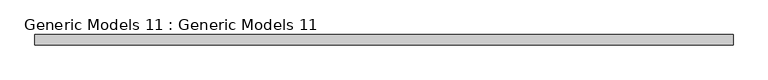
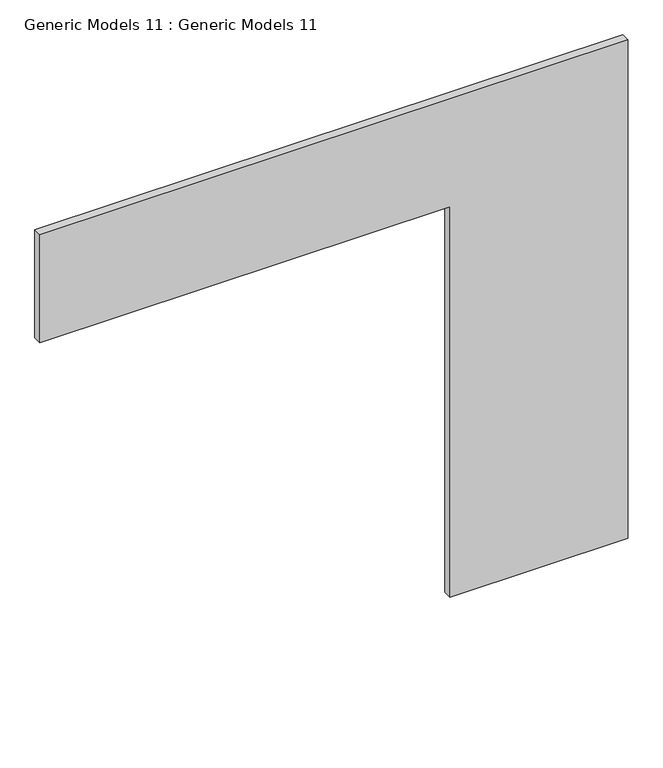
"""IFC4 building model written with IfcOpenShell, lengths in millimetres: proxy geometry, Generic Models 11 : Generic Models 11."""

from ifc_helpers import new_model, si_unit, frame, origin, place, context, project, spatial, polyline, outline, extrude, source, transform, mapped, element, save


def generic_models_11_generic_models_11_47c1f207(model_context):
    return source(origin(), model_context, "Body", "SweptSolid", [
        extrude(outline(polyline([(3352.8, -2406.7607439), (3352.8, -5810.3607439), (2692.4, -5810.3607439), (2692.4, -3435.4607439), (304.8, -3435.4607439), (304.8, -2406.7607439), (2673.920695, -2406.7607439), (3352.8, -2406.7607439)])), frame((0.0, -6621.2842658, 0.0), z_axis=(0.0, 1.0, 0.0), x_axis=(0.0, 0.0, 1.0)), (0.0, 0.0, 1.0), 50.8),
    ])


if __name__ == "__main__":
    model = new_model("IFC4")
    model_context = context("Model", 3, world=origin())
    ifc_project = project(units=[si_unit("LENGTHUNIT", "METRE", prefix="MILLI")], contexts=[model_context])
    site = spatial("IfcSite", under=ifc_project)
    building = spatial("IfcBuilding", under=site)
    placement = place(None, origin())
    generic_models_11_generic_models_11_shape = generic_models_11_generic_models_11_47c1f207(model_context)
    element("IfcBuildingElementProxy", 1, Name="Generic Models 11 : Generic Models 11", ObjectType="Generic Models 11 : Generic Models 11", at=placement, inside=building, context=model_context, shape_type="MappedRepresentation", body=[
        mapped(generic_models_11_generic_models_11_shape, transform((0.0, 0.0, 0.0), x_axis=(1.0, 0.0, 0.0), y_axis=(0.0, 1.0, 0.0), z_axis=(0.0, 0.0, 1.0))),
    ])
    save(model, "model.ifc")

# Revit data of these elements
# Element 1 (IfcBuildingElementProxy, "Generic Models 11 : Generic Models 11")
#   Materials on its faces: "CLADDING WALL MATERIAL"
# Materials
#   "CLADDING WALL MATERIAL": class "Generic", colour RGB 120 120 120, transparency 0, Cost = 0
